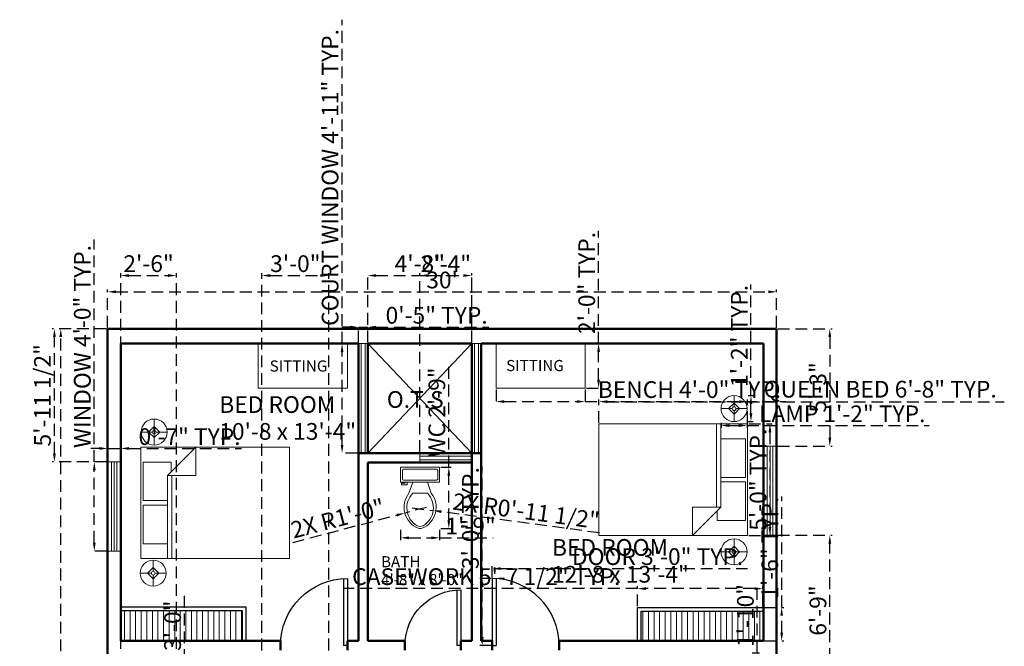
# Model space of a CAD drawing. Units: inches. Extents: x 3209 to 7144, y 1281 to 3076.
# Tile 4 of 5: x 3229 to 3758, y 1680 to 2018. Entities that reach past the tile are written whole.
import ezdxf

# ---------------------------------------------------------------- set-up
doc = ezdxf.new("R2010")
doc.units = ezdxf.units.IN
doc.linetypes.add('HIDDEN', pattern=[9.525, 6.35, -3.175])
for name, color, linetype, lineweight in [('A-ANNO-DIMS', 244, 'HIDDEN', 18), ('A-AREA-IDEN', 7, 'Continuous', 25), ('A-DOOR', 4, 'Continuous', 25), ('A-FLOR-CASE', 8, 'Continuous', 25), ('A-FLOR-CASE-PATT', 252, 'Continuous', 13), ('A-FLOR-FIXT', 9, 'Continuous', 18), ('A-FLOR-OPEN', 8, 'Continuous', 13), ('A-FURN', 8, 'Continuous', 18), ('A-GLAZ', 4, 'Continuous', 18), ('A-WALL', 7, 'Continuous', 50)]:
    doc.layers.add(name, color=color, linetype=linetype, lineweight=lineweight)
doc.styles.get("Standard").update_dxf_attribs({"font": 'arial.ttf'})
doc.dimstyles.new('ISO-25', dxfattribs={"dimtxt": 9, "dimasz": 4.5, "dimexe": 1.25, "dimexo": 0.625, "dimtad": 1, "dimdec": 0, "dimlunit": 3, "dimtxsty": 'Standard', "dimcen": 2.5, "dimadec": 0, "dimazin": 0, "dimtfac": 1, "dimtdec": 0, "dimtmove": 0, "dimatfit": 3, "dimfxl": 1, "dimarcsym": 0})

# ---------------------------------------------------------------- blocks, each defined once
blk = doc.blocks.new('Toilet - top')
for p, q in [((9.5, -6), (9.5, -2)), ((-10, -8.5), (-8, -8.5)), ((-10, -9.5), (-10, -8.5)), ((-7, -9.5), (-10, -9.5)), ((-8, -8.5), (-8, -8)), ((-7, -8), (-7, -9.5)), ((-4, -8), (-6, -14)), ((4, -8), (6, -14)), ((4, -14), (-4, -14))]:
    blk.add_line(p, q)
blk.add_lwpolyline([(10.5, -8), (10.5, 0), (-10.5, 0), (-10.5, -8)], close=True)
for points in [[(-9.5, -2), (-9.5, -6)], [(8.5, -1), (-8.5, -1)], [(-8.5, -7), (8.5, -7)]]:
    blk.add_lwpolyline(points)
for centre, radius, start, end in [((-8.62, -1.88), 0.884, 81.8699, 188.1301), ((8.62, -1.88), 0.884, 351.8699, 98.1301), ((-8.62, -6.12), 0.884, 171.8699, 278.1301), ((8.62, -6.12), 0.884, 261.8699, 8.1301), ((3.52, -21.58), 12.17, 141.4691, 247.9714), ((4.2, -21.82), 11.33, 136.3677, 238.9468), ((-3.52, -21.58), 12.17, 292.0284, 38.5307), ((-4.2, -21.82), 11.33, 301.053, 43.6321), ((0, -27.88), 4, 245.7318, 294.2682), ((0, -29), 4, 254.8605, 285.1395)]:
    blk.add_arc(centre, radius, start, end)
blk = doc.blocks.new('Bed - Queen')
for p, q in [((0, -80.00003), (0, 0)), ((0, 0), (59.99999, 0)), ((59.99999, 0), (59.99999, -80.00003)), ((7.99999, -1.2), (28.79998, -1.2)), ((7.99999, -14.4), (7.99999, -1.2)), ((28.79998, -1.2), (28.79998, -14.4)), ((31.19999, -1.2), (51.99999, -1.2)), ((31.19999, -14.4), (31.19999, -1.2)), ((51.99999, -1.2), (51.99999, -16.4)), ((0, -14.4), (44.8, -14.4)), ((59.99999, -29.6), (44.8, -14.4)), ((44.8, -14.4), (44.8, -29.6)), ((44.8, -16.8), (0, -16.8)), ((51.99999, -16.4), (46.79936, -16.4)), ((44.8, -29.6), (59.99999, -29.6)), ((59.99999, -80.00003), (0, -80.00003))]:
    blk.add_line(p, q)
blk = doc.blocks.new('Lamp - Table')
for p, q in [((0, 7), (0, 1)), ((-1, 0), (-7, 0)), ((0, 3), (-3, 0)), ((-3, 0), (0, -3)), ((3, 0), (0, 3)), ((0, -3), (3, 0)), ((1, 0), (7, 0)), ((0, -1), (0, -7))]:
    blk.add_line(p, q)
for radius in [7, 1]:
    blk.add_circle((0, 0), radius)
blk = doc.blocks.new('*D15')
at = {"layer": 'A-ANNO-DIMS', "color": 0, "lineweight": -2, "transparency": 16777216}
for p, q in [((3275.31, 1851.27), (3249.46, 1851.27)), ((3250.71, 1315.77), (3250.71, 1846.77)), ((3275.31, 1311.27), (3249.46, 1311.27))]:
    blk.add_line(p, q, dxfattribs=at)
at = {"layer": 'A-ANNO-DIMS', "color": 0, "transparency": 16777216}
for points in [[(3249.96, 1846.77), (3251.46, 1846.77), (3250.71, 1851.27)], [(3249.96, 1315.77), (3251.46, 1315.77), (3250.71, 1311.27)]]:
    blk.add_solid(points, dxfattribs=at)
at = {"layer": 'Defpoints', "color": 0, "transparency": 16777216}
for p in [(3250.71, 1851.27), (3275.94, 1851.27), (3275.94, 1311.27)]:
    blk.add_point(p, dxfattribs=at)
at = {"layer": 'A-ANNO-DIMS', "color": 0, "transparency": 16777216, "insert": (3245.51, 1581.27), "char_height": 9, "attachment_point": 5, "rotation": 90}
blk.add_mtext("45'", dxfattribs=at)
blk = doc.blocks.new('*D16')
at = {"layer": 'A-ANNO-DIMS', "color": 0, "lineweight": -2, "transparency": 16777216}
for p, q in [((3275.94, 1851.89), (3275.94, 1872.38)), ((3280.44, 1871.13), (3631.44, 1871.13)), ((3635.94, 1851.89), (3635.94, 1872.38))]:
    blk.add_line(p, q, dxfattribs=at)
at = {"layer": 'A-ANNO-DIMS', "color": 0, "transparency": 16777216}
for points in [[(3280.44, 1871.88), (3280.44, 1870.38), (3275.94, 1871.13)], [(3631.44, 1871.88), (3631.44, 1870.38), (3635.94, 1871.13)]]:
    blk.add_solid(points, dxfattribs=at)
at = {"layer": 'Defpoints', "color": 0, "transparency": 16777216}
for p in [(3635.94, 1871.13), (3275.94, 1851.27), (3635.94, 1851.27)]:
    blk.add_point(p, dxfattribs=at)
at = {"layer": 'A-ANNO-DIMS', "color": 0, "transparency": 16777216, "insert": (3455.94, 1876.35), "char_height": 9, "attachment_point": 5}
blk.add_mtext("30'", dxfattribs=at)
blk = doc.blocks.new('DOOR-SWING-36IN')
for p, q in [((0, 36), (0, 0)), ((2, 36), (2, 0)), ((0, 0), (2, 0))]:
    blk.add_line(p, q)
blk.add_arc((0, 0), 36, 0, 90)
blk = doc.blocks.new('DOOR-SWING-30IN')
for p, q in [((30, 30), (0, 30)), ((0, 30), (0, 28)), ((30, 28), (0, 28))]:
    blk.add_line(p, q)
blk.add_arc((0, 30), 30, 270, 0)
blk = doc.blocks.new('BENCH-48X24IN')
for p, q in [((0, 0), (0, 24)), ((48, 0), (48, 24)), ((0, 0), (48, 0))]:
    blk.add_line(p, q)
blk = doc.blocks.new('WINDOW-48IN-WALL7')
for p, q in [((0, 48), (7, 48)), ((2, 48), (2, 0)), ((3.5, 48), (3.5, 0)), ((5, 48), (5, 0)), ((0, 0), (7, 0))]:
    blk.add_line(p, q)
blk = doc.blocks.new('CASEWORK-BEDROOM-SURROUND')
for p, q in [((0, 67.48), (18, 67.48)), ((0, 65.48), (16, 65.48)), ((16, 65.48), (16, 0)), ((18, 67.48), (18, 0))]:
    blk.add_line(p, q)
blk = doc.blocks.new('WINDOW-LIGHTCOURT-59IN')
for p, q in [((0, 59), (5, 59)), ((1.5, 0), (1.5, 59)), ((3.5, 0), (3.5, 59))]:
    blk.add_line(p, q)
blk = doc.blocks.new('*D24')
at = {"layer": 'A-ANNO-DIMS', "color": 0, "lineweight": -2, "transparency": 16777216}
for p, q in [((3606.05, 1800.65), (3606.05, 1797.92)), ((3610.55, 1799.17), (3615.55, 1799.17)), ((3620.05, 1800.65), (3620.05, 1797.92)), ((3620.05, 1799.17), (3717.99, 1799.17))]:
    blk.add_line(p, q, dxfattribs=at)
at = {"layer": 'A-ANNO-DIMS', "color": 0, "transparency": 16777216}
for points in [[(3610.55, 1799.92), (3610.55, 1798.42), (3606.05, 1799.17)], [(3615.55, 1799.92), (3615.55, 1798.42), (3620.05, 1799.17)]]:
    blk.add_solid(points, dxfattribs=at)
at = {"layer": 'Defpoints', "color": 0, "transparency": 16777216}
for p in [(3606.05, 1801.27), (3620.05, 1801.27), (3620.05, 1799.17)]:
    blk.add_point(p, dxfattribs=at)
at = {"layer": 'A-ANNO-DIMS', "color": 0, "transparency": 16777216, "insert": (3671.27, 1804.32), "char_height": 9, "attachment_point": 5}
blk.add_mtext('LAMP 1\'-2" TYP.', dxfattribs=at)
blk = doc.blocks.new('*D25')
at = {"layer": 'A-ANNO-DIMS', "color": 0, "lineweight": -2, "transparency": 16777216}
for p, q in [((3622.15, 1815.27), (3622.15, 1875.04)), ((3620.68, 1815.27), (3623.4, 1815.27)), ((3622.15, 1805.77), (3622.15, 1810.77)), ((3620.68, 1801.27), (3623.4, 1801.27))]:
    blk.add_line(p, q, dxfattribs=at)
at = {"layer": 'A-ANNO-DIMS', "color": 0, "transparency": 16777216}
for points in [[(3621.4, 1810.77), (3622.9, 1810.77), (3622.15, 1815.27)], [(3621.4, 1805.77), (3622.9, 1805.77), (3622.15, 1801.27)]]:
    blk.add_solid(points, dxfattribs=at)
at = {"layer": 'Defpoints', "color": 0, "transparency": 16777216}
for p in [(3620.05, 1815.27), (3622.15, 1815.27), (3620.05, 1801.27)]:
    blk.add_point(p, dxfattribs=at)
at = {"layer": 'A-ANNO-DIMS', "color": 0, "transparency": 16777216, "insert": (3617.01, 1847.41), "char_height": 9, "attachment_point": 5, "rotation": 90}
blk.add_mtext('1\'-2" TYP.', dxfattribs=at)
blk = doc.blocks.new('*D27')
at = {"layer": 'A-ANNO-DIMS', "color": 0, "lineweight": -2, "transparency": 16777216}
for p, q in [((3625.56, 1676.78), (3625.56, 1712.6)), ((3622.87, 1676.78), (3626.81, 1676.78)), ((3625.56, 1659.22), (3625.56, 1672.28)), ((3622.87, 1654.72), (3626.81, 1654.72))]:
    blk.add_line(p, q, dxfattribs=at)
at = {"layer": 'A-ANNO-DIMS', "color": 0, "transparency": 16777216}
for points in [[(3624.81, 1672.28), (3626.31, 1672.28), (3625.56, 1676.78)], [(3624.81, 1659.22), (3626.31, 1659.22), (3625.56, 1654.72)]]:
    blk.add_solid(points, dxfattribs=at)
at = {"layer": 'Defpoints', "color": 0, "transparency": 16777216}
for p in [(3622.25, 1676.78), (3625.56, 1676.78), (3622.25, 1654.72)]:
    blk.add_point(p, dxfattribs=at)
at = {"layer": 'A-ANNO-DIMS', "color": 0, "transparency": 16777216, "insert": (3620.34, 1696.94), "char_height": 9, "attachment_point": 5, "rotation": 90}
blk.add_mtext('1\'-10"', dxfattribs=at)
blk = doc.blocks.new('*D30')
at = {"layer": 'A-ANNO-DIMS', "color": 0, "lineweight": -2, "transparency": 16777216}
for p, q in [((3268.74, 1779.63), (3268.74, 1899.27)), ((3275.31, 1779.63), (3267.49, 1779.63)), ((3268.74, 1736.13), (3268.74, 1775.13)), ((3275.31, 1731.63), (3267.49, 1731.63))]:
    blk.add_line(p, q, dxfattribs=at)
at = {"layer": 'A-ANNO-DIMS', "color": 0, "transparency": 16777216}
for points in [[(3267.99, 1775.13), (3269.49, 1775.13), (3268.74, 1779.63)], [(3267.99, 1736.13), (3269.49, 1736.13), (3268.74, 1731.63)]]:
    blk.add_solid(points, dxfattribs=at)
at = {"layer": 'Defpoints', "color": 0, "transparency": 16777216}
for p in [(3268.74, 1779.63), (3275.94, 1779.63), (3275.94, 1731.63)]:
    blk.add_point(p, dxfattribs=at)
at = {"layer": 'A-ANNO-DIMS', "color": 0, "transparency": 16777216, "insert": (3263.46, 1841.7), "char_height": 9, "attachment_point": 5, "rotation": 90}
blk.add_mtext('WINDOW 4\'-0" TYP.', dxfattribs=at)
blk = doc.blocks.new('*D31')
at = {"layer": 'A-ANNO-DIMS', "color": 0, "lineweight": -2, "transparency": 16777216}
for p, q in [((3271.44, 1786.83), (3266.94, 1786.83)), ((3275.94, 1780.25), (3275.94, 1788.08)), ((3275.94, 1786.83), (3282.94, 1786.83)), ((3282.94, 1780.25), (3282.94, 1788.08)), ((3287.44, 1786.83), (3348.05, 1786.83))]:
    blk.add_line(p, q, dxfattribs=at)
at = {"layer": 'A-ANNO-DIMS', "color": 0, "transparency": 16777216}
for points in [[(3271.44, 1787.58), (3271.44, 1786.08), (3275.94, 1786.83)], [(3287.44, 1787.58), (3287.44, 1786.08), (3282.94, 1786.83)]]:
    blk.add_solid(points, dxfattribs=at)
at = {"layer": 'Defpoints', "color": 0, "transparency": 16777216}
for p in [(3282.94, 1786.83), (3275.94, 1779.63), (3282.94, 1779.63)]:
    blk.add_point(p, dxfattribs=at)
at = {"layer": 'A-ANNO-DIMS', "color": 0, "transparency": 16777216, "insert": (3319.99, 1792.05), "char_height": 9, "attachment_point": 5}
blk.add_mtext('0\'-7" TYP.', dxfattribs=at)
blk = doc.blocks.new('*D32')
at = {"layer": 'A-ANNO-DIMS', "color": 0, "lineweight": -2, "transparency": 16777216}
for p, q in [((3540.36, 1800.63), (3540.36, 1813.26)), ((3620.36, 1800.63), (3620.36, 1813.26)), ((3544.86, 1812.01), (3615.86, 1812.01)), ((3620.36, 1812.01), (3758.5, 1812.01))]:
    blk.add_line(p, q, dxfattribs=at)
at = {"layer": 'A-ANNO-DIMS', "color": 0, "transparency": 16777216}
for points in [[(3544.86, 1812.76), (3544.86, 1811.26), (3540.36, 1812.01)], [(3615.86, 1812.76), (3615.86, 1811.26), (3620.36, 1812.01)]]:
    blk.add_solid(points, dxfattribs=at)
at = {"layer": 'Defpoints', "color": 0, "transparency": 16777216}
for p in [(3620.36, 1812.01), (3540.36, 1800.01), (3620.36, 1800.01)]:
    blk.add_point(p, dxfattribs=at)
at = {"layer": 'A-ANNO-DIMS', "color": 0, "transparency": 16777216, "insert": (3691.68, 1817.56), "char_height": 9, "attachment_point": 5}
blk.add_mtext('QUEEN BED 6\'-8" TYP.', dxfattribs=at)
blk = doc.blocks.new('*D33')
at = {"layer": 'A-ANNO-DIMS', "color": 0, "lineweight": -2, "transparency": 16777216}
for p, q in [((3620.98, 1800.01), (3633.61, 1800.01)), ((3632.36, 1795.51), (3632.36, 1744.51)), ((3620.98, 1740.01), (3633.61, 1740.01))]:
    blk.add_line(p, q, dxfattribs=at)
at = {"layer": 'A-ANNO-DIMS', "color": 0, "transparency": 16777216}
for points in [[(3631.61, 1795.51), (3633.11, 1795.51), (3632.36, 1800.01)], [(3631.61, 1744.51), (3633.11, 1744.51), (3632.36, 1740.01)]]:
    blk.add_solid(points, dxfattribs=at)
at = {"layer": 'Defpoints', "color": 0, "transparency": 16777216}
for p in [(3620.36, 1800.01), (3620.36, 1740.01), (3632.36, 1740.01)]:
    blk.add_point(p, dxfattribs=at)
at = {"layer": 'A-ANNO-DIMS', "color": 0, "transparency": 16777216, "insert": (3627.14, 1770.01), "char_height": 9, "attachment_point": 5, "rotation": 90}
blk.add_mtext('5\'-0" TYP.', dxfattribs=at)
blk = doc.blocks.new('*D36')
at = {"layer": 'A-ANNO-DIMS', "color": 0, "lineweight": -2, "transparency": 16777216}
for p, q in [((3482.94, 1717.39), (3482.94, 1723.42)), ((3518.94, 1717.39), (3518.94, 1723.42)), ((3487.44, 1722.17), (3514.44, 1722.17)), ((3518.94, 1722.17), (3620.31, 1722.17))]:
    blk.add_line(p, q, dxfattribs=at)
at = {"layer": 'A-ANNO-DIMS', "color": 0, "transparency": 16777216}
for points in [[(3487.44, 1722.92), (3487.44, 1721.42), (3482.94, 1722.17)], [(3514.44, 1722.92), (3514.44, 1721.42), (3518.94, 1722.17)]]:
    blk.add_solid(points, dxfattribs=at)
at = {"layer": 'Defpoints', "color": 0, "transparency": 16777216}
for p in [(3518.94, 1722.17), (3482.94, 1716.77), (3518.94, 1716.77)]:
    blk.add_point(p, dxfattribs=at)
at = {"layer": 'A-ANNO-DIMS', "color": 0, "transparency": 16777216, "insert": (3571.87, 1727.45), "char_height": 9, "attachment_point": 5}
blk.add_mtext('DOOR 3\'-0" TYP.', dxfattribs=at)
blk = doc.blocks.new('*D37')
at = {"layer": 'A-ANNO-DIMS', "color": 0, "lineweight": -2, "transparency": 16777216}
for p, q in [((3477.54, 1716.77), (3477.54, 1777.37)), ((3482.31, 1716.77), (3476.29, 1716.77)), ((3477.54, 1685.27), (3477.54, 1712.27)), ((3482.31, 1680.77), (3476.29, 1680.77))]:
    blk.add_line(p, q, dxfattribs=at)
at = {"layer": 'A-ANNO-DIMS', "color": 0, "transparency": 16777216}
for points in [[(3476.79, 1712.27), (3478.29, 1712.27), (3477.54, 1716.77)], [(3476.79, 1685.27), (3478.29, 1685.27), (3477.54, 1680.77)]]:
    blk.add_solid(points, dxfattribs=at)
at = {"layer": 'Defpoints', "color": 0, "transparency": 16777216}
for p in [(3477.54, 1716.77), (3482.94, 1716.77), (3482.94, 1680.77)]:
    blk.add_point(p, dxfattribs=at)
at = {"layer": 'A-ANNO-DIMS', "color": 0, "transparency": 16777216, "insert": (3472.32, 1749.32), "char_height": 9, "attachment_point": 5, "rotation": 90}
blk.add_mtext('3\'-0" TYP.', dxfattribs=at)
blk = doc.blocks.new('*D38')
at = {"layer": 'A-ANNO-DIMS', "color": 0, "lineweight": -2, "transparency": 16777216}
for p, q in [((3561.08, 1701.89), (3561.08, 1712.64)), ((3628.56, 1701.89), (3628.56, 1712.64)), ((3561.08, 1711.39), (3402.76, 1711.39)), ((3624.06, 1711.39), (3565.58, 1711.39))]:
    blk.add_line(p, q, dxfattribs=at)
at = {"layer": 'A-ANNO-DIMS', "color": 0, "transparency": 16777216}
for points in [[(3565.58, 1712.14), (3565.58, 1710.64), (3561.08, 1711.39)], [(3624.06, 1712.14), (3624.06, 1710.64), (3628.56, 1711.39)]]:
    blk.add_solid(points, dxfattribs=at)
at = {"layer": 'Defpoints', "color": 0, "transparency": 16777216}
for p in [(3561.08, 1711.39), (3561.08, 1701.27), (3628.56, 1701.27)]:
    blk.add_point(p, dxfattribs=at)
at = {"layer": 'A-ANNO-DIMS', "color": 0, "transparency": 16777216, "insert": (3479.67, 1716.67), "char_height": 9, "attachment_point": 5}
blk.add_mtext('CASEWORK 5\'-7 1/2" TYP.', dxfattribs=at)
blk = doc.blocks.new('*D39')
at = {"layer": 'A-ANNO-DIMS', "color": 0, "lineweight": -2, "transparency": 16777216}
for p, q in [((3638.68, 1701.27), (3638.68, 1761.03)), ((3629.19, 1701.27), (3639.93, 1701.27)), ((3638.68, 1687.77), (3638.68, 1696.77)), ((3629.19, 1683.27), (3639.93, 1683.27))]:
    blk.add_line(p, q, dxfattribs=at)
at = {"layer": 'A-ANNO-DIMS', "color": 0, "transparency": 16777216}
for points in [[(3637.93, 1696.77), (3639.43, 1696.77), (3638.68, 1701.27)], [(3637.93, 1687.77), (3639.43, 1687.77), (3638.68, 1683.27)]]:
    blk.add_solid(points, dxfattribs=at)
at = {"layer": 'Defpoints', "color": 0, "transparency": 16777216}
for p in [(3628.56, 1701.27), (3638.68, 1701.27), (3628.56, 1683.27)]:
    blk.add_point(p, dxfattribs=at)
at = {"layer": 'A-ANNO-DIMS', "color": 0, "transparency": 16777216, "insert": (3633.46, 1733.4), "char_height": 9, "attachment_point": 5, "rotation": 90}
blk.add_mtext('1\'-6" TYP.', dxfattribs=at)
blk = doc.blocks.new('*D44')
at = {"layer": 'A-ANNO-DIMS', "color": 0, "lineweight": -2, "transparency": 16777216}
for p, q in [((3484.94, 1818.64), (3484.94, 1810.82)), ((3532.94, 1818.64), (3532.94, 1810.82)), ((3489.44, 1812.07), (3528.44, 1812.07)), ((3532.94, 1812.07), (3640.66, 1812.07))]:
    blk.add_line(p, q, dxfattribs=at)
at = {"layer": 'A-ANNO-DIMS', "color": 0, "transparency": 16777216}
for points in [[(3489.44, 1812.82), (3489.44, 1811.32), (3484.94, 1812.07)], [(3528.44, 1812.82), (3528.44, 1811.32), (3532.94, 1812.07)]]:
    blk.add_solid(points, dxfattribs=at)
at = {"layer": 'Defpoints', "color": 0, "transparency": 16777216}
for p in [(3484.94, 1819.27), (3532.94, 1819.27), (3532.94, 1812.07)]:
    blk.add_point(p, dxfattribs=at)
at = {"layer": 'A-ANNO-DIMS', "color": 0, "transparency": 16777216, "insert": (3589.05, 1817.35), "char_height": 9, "attachment_point": 5}
blk.add_mtext('BENCH 4\'-0" TYP.', dxfattribs=at)
blk = doc.blocks.new('*D45')
at = {"layer": 'A-ANNO-DIMS', "color": 0, "lineweight": -2, "transparency": 16777216}
for p, q in [((3540.14, 1843.27), (3540.14, 1904.03)), ((3533.57, 1843.27), (3541.39, 1843.27)), ((3540.14, 1823.77), (3540.14, 1838.77)), ((3533.57, 1819.27), (3541.39, 1819.27))]:
    blk.add_line(p, q, dxfattribs=at)
at = {"layer": 'A-ANNO-DIMS', "color": 0, "transparency": 16777216}
for points in [[(3539.39, 1838.77), (3540.89, 1838.77), (3540.14, 1843.27)], [(3539.39, 1823.77), (3540.89, 1823.77), (3540.14, 1819.27)]]:
    blk.add_solid(points, dxfattribs=at)
at = {"layer": 'Defpoints', "color": 0, "transparency": 16777216}
for p in [(3532.94, 1843.27), (3540.14, 1843.27), (3532.94, 1819.27)]:
    blk.add_point(p, dxfattribs=at)
at = {"layer": 'A-ANNO-DIMS', "color": 0, "transparency": 16777216, "insert": (3534.92, 1875.9), "char_height": 9, "attachment_point": 5, "rotation": 90}
blk.add_mtext('2\'-0" TYP.', dxfattribs=at)
blk = doc.blocks.new('*D48')
at = {"layer": 'A-ANNO-DIMS', "color": 0, "lineweight": -2, "transparency": 16777216}
for p, q in [((3402.09, 1843.27), (3402.09, 2017.62)), ((3410.31, 1843.27), (3400.84, 1843.27)), ((3402.09, 1788.77), (3402.09, 1838.77)), ((3410.31, 1784.27), (3400.84, 1784.27))]:
    blk.add_line(p, q, dxfattribs=at)
at = {"layer": 'A-ANNO-DIMS', "color": 0, "transparency": 16777216}
for points in [[(3401.34, 1838.77), (3402.84, 1838.77), (3402.09, 1843.27)], [(3401.34, 1788.77), (3402.84, 1788.77), (3402.09, 1784.27)]]:
    blk.add_solid(points, dxfattribs=at)
at = {"layer": 'Defpoints', "color": 0, "transparency": 16777216}
for p in [(3402.09, 1843.27), (3410.94, 1843.27), (3410.94, 1784.27)]:
    blk.add_point(p, dxfattribs=at)
at = {"layer": 'A-ANNO-DIMS', "color": 0, "transparency": 16777216, "insert": (3396.81, 1932.69), "char_height": 9, "attachment_point": 5, "rotation": 90}
blk.add_mtext('COURT WINDOW 4\'-11" TYP.', dxfattribs=at)
blk = doc.blocks.new('*D49')
at = {"layer": 'A-ANNO-DIMS', "color": 0, "lineweight": -2, "transparency": 16777216}
for p, q in [((3406.44, 1852.12), (3401.94, 1852.12)), ((3410.94, 1843.89), (3410.94, 1853.37)), ((3410.94, 1852.12), (3415.94, 1852.12)), ((3415.94, 1843.89), (3415.94, 1853.37)), ((3420.44, 1852.12), (3481.05, 1852.12))]:
    blk.add_line(p, q, dxfattribs=at)
at = {"layer": 'A-ANNO-DIMS', "color": 0, "transparency": 16777216}
for points in [[(3406.44, 1852.87), (3406.44, 1851.37), (3410.94, 1852.12)], [(3420.44, 1852.87), (3420.44, 1851.37), (3415.94, 1852.12)]]:
    blk.add_solid(points, dxfattribs=at)
at = {"layer": 'Defpoints', "color": 0, "transparency": 16777216}
for p in [(3415.94, 1852.12), (3410.94, 1843.27), (3415.94, 1843.27)]:
    blk.add_point(p, dxfattribs=at)
at = {"layer": 'A-ANNO-DIMS', "color": 0, "transparency": 16777216, "insert": (3452.99, 1857.34), "char_height": 9, "attachment_point": 5}
blk.add_mtext('0\'-5" TYP.', dxfattribs=at)
blk = doc.blocks.new('*D50')
at = {"layer": 'A-ANNO-DIMS', "color": 0, "lineweight": -2, "transparency": 16777216}
for p, q in [((3459.55, 1776.72), (3459.55, 1831.21)), ((3455.22, 1776.72), (3460.8, 1776.72)), ((3459.55, 1748.18), (3459.55, 1772.22)), ((3455.22, 1743.68), (3460.8, 1743.68))]:
    blk.add_line(p, q, dxfattribs=at)
at = {"layer": 'A-ANNO-DIMS', "color": 0, "transparency": 16777216}
for points in [[(3458.8, 1772.22), (3460.3, 1772.22), (3459.55, 1776.72)], [(3458.8, 1748.18), (3460.3, 1748.18), (3459.55, 1743.68)]]:
    blk.add_solid(points, dxfattribs=at)
at = {"layer": 'Defpoints', "color": 0, "transparency": 16777216}
for p in [(3454.59, 1776.72), (3459.55, 1776.72), (3454.59, 1743.68)]:
    blk.add_point(p, dxfattribs=at)
at = {"layer": 'A-ANNO-DIMS', "color": 0, "transparency": 16777216, "insert": (3454.27, 1806.21), "char_height": 9, "attachment_point": 5, "rotation": 90}
blk.add_mtext('WC 2\'-9"', dxfattribs=at)
blk = doc.blocks.new('*D51')
at = {"layer": 'A-ANNO-DIMS', "color": 0, "lineweight": -2, "transparency": 16777216}
for p, q in [((3433.59, 1743.05), (3433.59, 1737.47)), ((3438.09, 1738.72), (3450.09, 1738.72)), ((3454.59, 1743.05), (3454.59, 1737.47)), ((3454.59, 1738.72), (3483.42, 1738.72))]:
    blk.add_line(p, q, dxfattribs=at)
at = {"layer": 'A-ANNO-DIMS', "color": 0, "transparency": 16777216}
for points in [[(3438.09, 1739.47), (3438.09, 1737.97), (3433.59, 1738.72)], [(3450.09, 1739.47), (3450.09, 1737.97), (3454.59, 1738.72)]]:
    blk.add_solid(points, dxfattribs=at)
at = {"layer": 'Defpoints', "color": 0, "transparency": 16777216}
for p in [(3433.59, 1743.68), (3454.59, 1743.68), (3454.59, 1738.72)]:
    blk.add_point(p, dxfattribs=at)
at = {"layer": 'A-ANNO-DIMS', "color": 0, "transparency": 16777216, "insert": (3471.26, 1743.94), "char_height": 9, "attachment_point": 5}
blk.add_mtext('1\'-9"', dxfattribs=at)
blk = doc.blocks.new('*D60')
at = {"layer": 'A-ANNO-DIMS', "color": 0, "lineweight": -2, "transparency": 16777216}
for p, q in [((3317.34, 1577.27), (3317.34, 1709.86)), ((3312.56, 1577.27), (3318.59, 1577.27)), ((3317.34, 1545.77), (3317.34, 1572.77)), ((3312.56, 1541.27), (3318.59, 1541.27))]:
    blk.add_line(p, q, dxfattribs=at)
at = {"layer": 'A-ANNO-DIMS', "color": 0, "transparency": 16777216}
for points in [[(3316.59, 1572.77), (3318.09, 1572.77), (3317.34, 1577.27)], [(3316.59, 1545.77), (3318.09, 1545.77), (3317.34, 1541.27)]]:
    blk.add_solid(points, dxfattribs=at)
at = {"layer": 'Defpoints', "color": 0, "transparency": 16777216}
for p in [(3311.94, 1577.27), (3317.34, 1577.27), (3311.94, 1541.27)]:
    blk.add_point(p, dxfattribs=at)
at = {"layer": 'A-ANNO-DIMS', "color": 0, "transparency": 16777216, "insert": (3312.05, 1645.82), "char_height": 9, "attachment_point": 5, "rotation": 90}
blk.add_mtext('REFRIGERATOR 3\'-0"', dxfattribs=at)
blk = doc.blocks.new('*D74')
at = {"layer": 'A-ANNO-DIMS', "color": 0, "lineweight": -2, "transparency": 16777216}
for p, q in [((3282.94, 1678.89), (3282.94, 1881.16)), ((3312.94, 1678.89), (3312.94, 1881.16)), ((3287.44, 1879.91), (3308.44, 1879.91))]:
    blk.add_line(p, q, dxfattribs=at)
at = {"layer": 'A-ANNO-DIMS', "color": 0, "transparency": 16777216}
for points in [[(3287.44, 1880.66), (3287.44, 1879.16), (3282.94, 1879.91)], [(3308.44, 1880.66), (3308.44, 1879.16), (3312.94, 1879.91)]]:
    blk.add_solid(points, dxfattribs=at)
at = {"layer": 'Defpoints', "color": 0, "transparency": 16777216}
for p in [(3312.94, 1879.91), (3282.94, 1678.27), (3312.94, 1678.27)]:
    blk.add_point(p, dxfattribs=at)
at = {"layer": 'A-ANNO-DIMS', "color": 0, "transparency": 16777216, "insert": (3297.94, 1885.14), "char_height": 9, "attachment_point": 5}
blk.add_mtext('2\'-6"', dxfattribs=at)
blk = doc.blocks.new('*D75')
at = {"layer": 'A-ANNO-DIMS', "color": 0, "lineweight": -2, "transparency": 16777216}
for p, q in [((3358.94, 1582.89), (3358.94, 1881.16)), ((3394.94, 1582.89), (3394.94, 1881.16)), ((3363.44, 1879.91), (3390.44, 1879.91))]:
    blk.add_line(p, q, dxfattribs=at)
at = {"layer": 'A-ANNO-DIMS', "color": 0, "transparency": 16777216}
for points in [[(3363.44, 1880.66), (3363.44, 1879.16), (3358.94, 1879.91)], [(3390.44, 1880.66), (3390.44, 1879.16), (3394.94, 1879.91)]]:
    blk.add_solid(points, dxfattribs=at)
at = {"layer": 'Defpoints', "color": 0, "transparency": 16777216}
for p in [(3394.94, 1879.91), (3358.94, 1582.27), (3394.94, 1582.27)]:
    blk.add_point(p, dxfattribs=at)
at = {"layer": 'A-ANNO-DIMS', "color": 0, "transparency": 16777216, "insert": (3376.94, 1885.14), "char_height": 9, "attachment_point": 5}
blk.add_mtext('3\'-0"', dxfattribs=at)
blk = doc.blocks.new('*D76')
at = {"layer": 'A-ANNO-DIMS', "color": 0, "lineweight": -2, "transparency": 16777216}
for p, q in [((3415.94, 1843.89), (3415.94, 1881.16)), ((3471.94, 1843.89), (3471.94, 1881.16)), ((3420.44, 1879.91), (3467.44, 1879.91))]:
    blk.add_line(p, q, dxfattribs=at)
at = {"layer": 'A-ANNO-DIMS', "color": 0, "transparency": 16777216}
for points in [[(3420.44, 1880.66), (3420.44, 1879.16), (3415.94, 1879.91)], [(3467.44, 1880.66), (3467.44, 1879.16), (3471.94, 1879.91)]]:
    blk.add_solid(points, dxfattribs=at)
at = {"layer": 'Defpoints', "color": 0, "transparency": 16777216}
for p in [(3471.94, 1879.91), (3415.94, 1843.27), (3471.94, 1843.27)]:
    blk.add_point(p, dxfattribs=at)
at = {"layer": 'A-ANNO-DIMS', "color": 0, "transparency": 16777216, "insert": (3443.94, 1885.14), "char_height": 9, "attachment_point": 5}
blk.add_mtext('4\'-8"', dxfattribs=at)
blk = doc.blocks.new('*D77')
at = {"layer": 'A-ANNO-DIMS', "color": 0, "lineweight": -2, "transparency": 16777216}
for p, q in [((3443.94, 1784.89), (3443.94, 1881.16)), ((3471.94, 1784.89), (3471.94, 1881.16)), ((3448.44, 1879.91), (3467.44, 1879.91))]:
    blk.add_line(p, q, dxfattribs=at)
at = {"layer": 'A-ANNO-DIMS', "color": 0, "transparency": 16777216}
for points in [[(3448.44, 1880.66), (3448.44, 1879.16), (3443.94, 1879.91)], [(3467.44, 1880.66), (3467.44, 1879.16), (3471.94, 1879.91)]]:
    blk.add_solid(points, dxfattribs=at)
at = {"layer": 'Defpoints', "color": 0, "transparency": 16777216}
for p in [(3471.94, 1879.91), (3443.94, 1784.27), (3471.94, 1784.27)]:
    blk.add_point(p, dxfattribs=at)
at = {"layer": 'A-ANNO-DIMS', "color": 0, "transparency": 16777216, "insert": (3457.94, 1885.06), "char_height": 9, "attachment_point": 5}
blk.add_mtext('2\'-4"', dxfattribs=at)
blk = doc.blocks.new('*D78')
at = {"layer": 'A-ANNO-DIMS', "color": 0, "lineweight": -2, "transparency": 16777216}
for p, q in [((3636.56, 1851.27), (3665.83, 1851.27)), ((3664.58, 1846.77), (3664.58, 1792.63)), ((3636.56, 1788.13), (3665.83, 1788.13))]:
    blk.add_line(p, q, dxfattribs=at)
at = {"layer": 'A-ANNO-DIMS', "color": 0, "transparency": 16777216}
for points in [[(3663.83, 1846.77), (3665.33, 1846.77), (3664.58, 1851.27)], [(3663.83, 1792.63), (3665.33, 1792.63), (3664.58, 1788.13)]]:
    blk.add_solid(points, dxfattribs=at)
at = {"layer": 'Defpoints', "color": 0, "transparency": 16777216}
for p in [(3635.94, 1851.27), (3635.94, 1788.13), (3664.58, 1788.13)]:
    blk.add_point(p, dxfattribs=at)
at = {"layer": 'A-ANNO-DIMS', "color": 0, "transparency": 16777216, "insert": (3659.36, 1819.7), "char_height": 9, "attachment_point": 5, "rotation": 90}
blk.add_mtext('5\'-3"', dxfattribs=at)
blk = doc.blocks.new('*D79')
at = {"layer": 'A-ANNO-DIMS', "color": 0, "lineweight": -2, "transparency": 16777216}
for p, q in [((3636.56, 1740.13), (3665.83, 1740.13)), ((3664.58, 1663.54), (3664.58, 1735.63)), ((3636.56, 1659.04), (3665.83, 1659.04))]:
    blk.add_line(p, q, dxfattribs=at)
at = {"layer": 'A-ANNO-DIMS', "color": 0, "transparency": 16777216}
for points in [[(3663.83, 1735.63), (3665.33, 1735.63), (3664.58, 1740.13)], [(3663.83, 1663.54), (3665.33, 1663.54), (3664.58, 1659.04)]]:
    blk.add_solid(points, dxfattribs=at)
at = {"layer": 'Defpoints', "color": 0, "transparency": 16777216}
for p in [(3635.94, 1740.13), (3664.58, 1740.13), (3635.94, 1659.04)]:
    blk.add_point(p, dxfattribs=at)
at = {"layer": 'A-ANNO-DIMS', "color": 0, "transparency": 16777216, "insert": (3659.36, 1699.59), "char_height": 9, "attachment_point": 5, "rotation": 90}
blk.add_mtext('6\'-9"', dxfattribs=at)
blk = doc.blocks.new('*D81')
at = {"layer": 'A-ANNO-DIMS', "color": 0, "lineweight": -2, "transparency": 16777216}
for p, q in [((3275.31, 1851.27), (3246.04, 1851.27)), ((3247.29, 1784.13), (3247.29, 1846.77)), ((3275.31, 1779.63), (3246.04, 1779.63))]:
    blk.add_line(p, q, dxfattribs=at)
at = {"layer": 'A-ANNO-DIMS', "color": 0, "transparency": 16777216}
for points in [[(3246.54, 1846.77), (3248.04, 1846.77), (3247.29, 1851.27)], [(3246.54, 1784.13), (3248.04, 1784.13), (3247.29, 1779.63)]]:
    blk.add_solid(points, dxfattribs=at)
at = {"layer": 'Defpoints', "color": 0, "transparency": 16777216}
for p in [(3247.29, 1851.27), (3275.94, 1851.27), (3275.94, 1779.63)]:
    blk.add_point(p, dxfattribs=at)
at = {"layer": 'A-ANNO-DIMS', "color": 0, "transparency": 16777216, "insert": (3242.01, 1815.45), "char_height": 9, "attachment_point": 5, "rotation": 90}
blk.add_mtext('5\'-11 1/2"', dxfattribs=at)
blk = doc.blocks.new('*D86')
at = {"layer": 'A-ANNO-DIMS', "color": 0, "lineweight": -2, "transparency": 16777216}
for p, q in [((3447.61, 1755.14), (3435.84, 1752.05)), ((3375.61, 1736.22), (3431.49, 1750.91))]:
    blk.add_line(p, q, dxfattribs=at)
at = {"layer": 'A-ANNO-DIMS', "color": 0, "transparency": 16777216}
blk.add_solid([(3431.3, 1751.63), (3431.68, 1750.18), (3435.84, 1752.05)], dxfattribs=at)
at = {"layer": 'Defpoints', "color": 0, "transparency": 16777216}
for p in [(3447.61, 1755.14), (3435.84, 1752.05)]:
    blk.add_point(p, dxfattribs=at)
at = {"layer": 'A-ANNO-DIMS', "color": 0, "transparency": 16777216, "insert": (3400.05, 1748.04), "char_height": 9, "attachment_point": 5, "rotation": 14.7213}
blk.add_mtext('2X R1\'-0"', dxfattribs=at)
blk = doc.blocks.new('*D87')
at = {"layer": 'A-ANNO-DIMS', "color": 0, "lineweight": -2, "transparency": 16777216}
for p, q in [((3439.89, 1754.91), (3451.12, 1753.4)), ((3540.56, 1741.37), (3455.58, 1752.8))]:
    blk.add_line(p, q, dxfattribs=at)
at = {"layer": 'A-ANNO-DIMS', "color": 0, "transparency": 16777216}
blk.add_solid([(3455.68, 1753.54), (3455.48, 1752.05), (3451.12, 1753.4)], dxfattribs=at)
at = {"layer": 'Defpoints', "color": 0, "transparency": 16777216}
for p in [(3439.89, 1754.91), (3451.12, 1753.4)]:
    blk.add_point(p, dxfattribs=at)
at = {"layer": 'A-ANNO-DIMS', "color": 0, "transparency": 16777216, "insert": (3501, 1752.02), "char_height": 9, "attachment_point": 5, "rotation": 352.3429}
blk.add_mtext('2X R0\'-11 1/2"', dxfattribs=at)

msp = doc.modelspace()

# ---------------------------------------------------------------- hatches: boundary and pattern name
at = {"layer": 'A-FLOR-CASE-PATT'}
h = msp.add_hatch(dxfattribs=at)
h.set_pattern_fill('ANSI31', color=256, scale=0.944882, angle=45, style=0)
h.paths.add_polyline_path([(3282.42, 1683.42), (3348.42, 1683.42), (3348.42, 1699.42), (3282.42, 1699.42)])
h = msp.add_hatch(dxfattribs=at)
h.set_pattern_fill('ANSI31', color=256, scale=0.944882, angle=45, style=0)
h.paths.add_polyline_path([(3563.08, 1683.27), (3628.56, 1683.27), (3628.56, 1699.27), (3563.08, 1699.27)])

# ---------------------------------------------------------------- linework, layer by layer
at = {"layer": 'A-FLOR-OPEN'}
for p, q in [((3415.94, 1843.27), (3471.94, 1784.27)), ((3415.94, 1784.27), (3471.94, 1843.27))]:
    msp.add_line(p, q, dxfattribs=at)
at = {"layer": 'A-GLAZ'}
for p, q in [((3443.94, 1784.27), (3443.94, 1779.27)), ((3443.94, 1782.77), (3471.94, 1782.77)), ((3443.94, 1780.77), (3471.94, 1780.77))]:
    msp.add_line(p, q, dxfattribs=at)
at = {"layer": 'A-WALL'}
for p, q in [((3275.94, 1851.27), (3635.94, 1851.27)), ((3275.94, 1311.27), (3275.94, 1851.27)), ((3635.94, 1851.27), (3635.94, 1311.27)), ((3282.94, 1843.27), (3410.94, 1843.27)), ((3282.94, 1683.27), (3282.94, 1843.27)), ((3410.94, 1683.27), (3410.94, 1843.27)), ((3415.94, 1784.27), (3415.94, 1843.27)), ((3415.94, 1843.27), (3471.94, 1843.27)), ((3471.94, 1843.27), (3471.94, 1779.27)), ((3476.94, 1843.27), (3476.94, 1683.27)), ((3476.94, 1843.27), (3628.94, 1843.27)), ((3628.94, 1843.27), (3628.94, 1683.27)), ((3410.94, 1784.27), (3476.94, 1784.27)), ((3415.94, 1683.27), (3415.94, 1779.27)), ((3415.94, 1779.27), (3471.94, 1779.27)), ((3471.94, 1779.27), (3471.94, 1683.27)), ((3282.94, 1683.27), (3368.94, 1683.27)), ((3368.94, 1678.27), (3368.94, 1683.27)), ((3404.94, 1683.27), (3410.94, 1683.27)), ((3404.94, 1678.27), (3404.94, 1683.27)), ((3415.94, 1683.27), (3435.94, 1683.27)), ((3435.94, 1683.27), (3435.94, 1678.27)), ((3465.94, 1683.27), (3465.94, 1678.27)), ((3465.94, 1683.27), (3471.94, 1683.27)), ((3476.94, 1683.27), (3482.94, 1683.27)), ((3482.94, 1683.27), (3482.94, 1678.27)), ((3518.94, 1683.27), (3518.94, 1678.27)), ((3518.94, 1683.27), (3628.94, 1683.27))]:
    msp.add_line(p, q, dxfattribs=at)

# ---------------------------------------------------------------- block references
at = {"layer": 'A-DOOR', "extrusion": (0, 0, -1), "zscale": -1}
msp.add_blockref('DOOR-SWING-36IN', (-3404.94, 1680.77), dxfattribs=at)
at = {"layer": 'A-DOOR'}
msp.add_blockref('DOOR-SWING-36IN', (3482.94, 1680.77), dxfattribs=at)
at = {"layer": 'A-DOOR', "extrusion": (0, 0, -1), "zscale": -1, "rotation": 90.0000000000039}
msp.add_blockref('DOOR-SWING-30IN', (-3435.94, 1680.77), dxfattribs=at)
at = {"layer": 'A-FLOR-CASE', "extrusion": (0, 0, -1), "zscale": -1, "rotation": 90.00000000000026}
msp.add_blockref('CASEWORK-BEDROOM-SURROUND', (-3282.94, 1683.42), dxfattribs=at)
at = {"layer": 'A-FLOR-CASE', "rotation": 90.00000000000055}
msp.add_blockref('CASEWORK-BEDROOM-SURROUND', (3628.56, 1683.27), dxfattribs=at)
at = {"layer": 'A-FLOR-FIXT'}
msp.add_blockref('Toilet - top', (3444.09, 1776.72), dxfattribs=at)
at = {"layer": 'A-FURN'}
for name, p in [('BENCH-48X24IN', (3356.94, 1819.27)), ('BENCH-48X24IN', (3484.94, 1819.27)), ('Lamp - Table', (3613.05, 1808.27)), ('Lamp - Table', (3300.97, 1795.66)), ('Lamp - Table', (3613.05, 1731.19)), ('Lamp - Table', (3300.45, 1719.7))]:
    msp.add_blockref(name, p, dxfattribs=at)
for p, rotation in [((3620.36, 1800.01), 270), ((3293.76, 1727.54), 90)]:
    msp.add_blockref('Bed - Queen', p, dxfattribs=dict(at, rotation=rotation))
at = {"layer": 'A-GLAZ'}
for name, p in [('WINDOW-LIGHTCOURT-59IN', (3410.94, 1784.27)), ('WINDOW-LIGHTCOURT-59IN', (3471.94, 1784.27)), ('WINDOW-48IN-WALL7', (3628.94, 1740.13)), ('WINDOW-48IN-WALL7', (3275.94, 1731.63))]:
    msp.add_blockref(name, p, dxfattribs=at)

# ---------------------------------------------------------------- texts
at = {"layer": 'A-AREA-IDEN'}
for s, height, p in [('SITTING ', 6, (3363.12, 1828.21)), ('SITTING ', 6, (3490.4, 1828.46)), ('O.T.S', 9, (3426.17, 1808.7)), ('BED ROOM ', 9, (3336, 1805.97)), ('10\'-8 x 13\'-4"', 9, (3336, 1791.51)), ('BED ROOM ', 9, (3515.07, 1729.07)), ('BATH', 6, (3423.05, 1722.87)), ('12\'-8 x 13\'-4"', 9, (3515.07, 1714.61)), ('4\'-8" x 8\'-0"', 6, (3423.05, 1713.24))]:
    msp.add_text(s, height=height, dxfattribs=at).set_placement(p)

# ---------------------------------------------------------------- dimensions: what is measured, and where the dimension line sits
at = {"layer": 'A-ANNO-DIMS'}
for base, p1, p2, angle, text, picture, middle in [((3402.09, 1843.27), (3410.94, 1784.27), (3410.94, 1843.27), 90, 'COURT WINDOW <> TYP.', '*D48', (3396.81, 1932.69)), ((3540.14, 1843.27), (3532.94, 1819.27), (3532.94, 1843.27), 90, '<> TYP.', '*D45', (3534.92, 1875.9)), ((3268.74, 1779.63), (3275.94, 1731.63), (3275.94, 1779.63), 90, 'WINDOW <> TYP.', '*D30', (3263.46, 1841.7)), ((3622.15, 1815.27), (3620.05, 1801.27), (3620.05, 1815.27), 90, '<> TYP.', '*D25', (3617.01, 1847.41)), ((3459.55, 1776.72), (3454.59, 1743.68), (3454.59, 1776.72), 90, 'WC <>', '*D50', (3454.27, 1806.21)), ((3632.36, 1740.01), (3620.36, 1800.01), (3620.36, 1740.01), 270, '<> TYP.', '*D33', (3627.14, 1770.01)), ((3477.54, 1716.77), (3482.94, 1680.77), (3482.94, 1716.77), 90, '<> TYP.', '*D37', (3472.32, 1749.32)), ((3638.68, 1701.27), (3628.56, 1683.27), (3628.56, 1701.27), 90, '<> TYP.', '*D39', (3633.46, 1733.4)), ((3561.08, 1711.39), (3628.56, 1701.27), (3561.08, 1701.27), 180, 'CASEWORK <> TYP.', '*D38', (3479.67, 1716.67)), ((3317.34, 1577.27), (3311.94, 1541.27), (3311.94, 1577.27), 90, 'REFRIGERATOR <>', '*D60', (3312.05, 1645.82))]:
    dim = msp.add_linear_dim(base=base, p1=p1, p2=p2, angle=angle, text=text, dimstyle='ISO-25', override={"dimdec": 1, "dimlfac": 1, "dimrnd": 0, "dimzin": 1, "dimdsep": 46, "dimlunit": 4, "dimfrac": 2}, dxfattribs=at)
    dim.commit()
    dim.dimension.update_dxf_attribs({"geometry": picture, "text_midpoint": middle})
for base, p1, p2, override, picture, middle in [((3312.94, 1879.91), (3282.94, 1678.27), (3312.94, 1678.27), {"dimdec": 1, "dimlfac": 1, "dimrnd": 0, "dimzin": 1, "dimdsep": 46, "dimlunit": 4, "dimfrac": 2}, '*D74', (3297.94, 1885.14)), ((3394.94, 1879.91), (3358.94, 1582.27), (3394.94, 1582.27), {"dimdec": 1, "dimlfac": 1, "dimrnd": 0, "dimzin": 1, "dimdsep": 46, "dimlunit": 4, "dimfrac": 2}, '*D75', (3376.94, 1885.14)), ((3471.94, 1879.91), (3415.94, 1843.27), (3471.94, 1843.27), {"dimdec": 1, "dimlfac": 1, "dimrnd": 0, "dimzin": 1, "dimdsep": 46, "dimlunit": 4, "dimfrac": 2}, '*D76', (3443.94, 1885.14)), ((3471.94, 1879.91), (3443.94, 1784.27), (3471.94, 1784.27), {"dimdec": 1, "dimlfac": 1, "dimrnd": 0, "dimzin": 1, "dimdsep": 46, "dimlunit": 4, "dimfrac": 2}, '*D77', (3457.94, 1885.06)), ((3635.94, 1871.13), (3275.94, 1851.27), (3635.94, 1851.27), {"dimclrd": 0, "dimclre": 0, "dimclrt": 0}, '*D16', (3455.94, 1876.35)), ((3454.59, 1738.72), (3433.59, 1743.68), (3454.59, 1743.68), {"dimdec": 1, "dimlfac": 1, "dimrnd": 0, "dimzin": 1, "dimdsep": 46, "dimlunit": 4, "dimfrac": 2}, '*D51', (3471.26, 1743.94))]:
    dim = msp.add_linear_dim(base=base, p1=p1, p2=p2, dimstyle='ISO-25', override=override, dxfattribs=at)
    dim.commit()
    dim.dimension.update_dxf_attribs({"geometry": picture, "text_midpoint": middle})
for base, p1, p2, text, picture, middle in [((3415.94, 1852.12), (3410.94, 1843.27), (3415.94, 1843.27), '<> TYP.', '*D49', (3452.99, 1857.34)), ((3620.36, 1812.01), (3540.36, 1800.01), (3620.36, 1800.01), 'QUEEN BED <> TYP.', '*D32', (3691.68, 1817.56)), ((3532.94, 1812.07), (3484.94, 1819.27), (3532.94, 1819.27), 'BENCH <> TYP.', '*D44', (3589.05, 1817.35)), ((3620.05, 1799.17), (3606.05, 1801.27), (3620.05, 1801.27), 'LAMP <> TYP.', '*D24', (3671.27, 1804.32)), ((3282.94, 1786.83), (3275.94, 1779.63), (3282.94, 1779.63), '<> TYP.', '*D31', (3319.99, 1792.05)), ((3518.94, 1722.17), (3482.94, 1716.77), (3518.94, 1716.77), 'DOOR <> TYP.', '*D36', (3571.87, 1727.45))]:
    dim = msp.add_linear_dim(base=base, p1=p1, p2=p2, text=text, dimstyle='ISO-25', override={"dimdec": 1, "dimlfac": 1, "dimrnd": 0, "dimzin": 1, "dimdsep": 46, "dimlunit": 4, "dimfrac": 2}, dxfattribs=at)
    dim.commit()
    dim.dimension.update_dxf_attribs({"geometry": picture, "text_midpoint": middle})
for base, p1, p2, override, picture, middle in [((3247.29, 1851.27), (3275.94, 1779.63), (3275.94, 1851.27), {"dimdec": 1, "dimlfac": 1, "dimrnd": 0, "dimzin": 1, "dimdsep": 46, "dimlunit": 4, "dimfrac": 2}, '*D81', (3242.01, 1815.45)), ((3250.71, 1851.27), (3275.94, 1311.27), (3275.94, 1851.27), {"dimclrd": 0, "dimclre": 0, "dimclrt": 0}, '*D15', (3245.51, 1581.27)), ((3664.58, 1788.13), (3635.94, 1851.27), (3635.94, 1788.13), {"dimdec": 1, "dimlfac": 1, "dimrnd": 0, "dimzin": 1, "dimdsep": 46, "dimlunit": 4, "dimfrac": 2}, '*D78', (3659.36, 1819.7)), ((3664.58, 1740.13), (3635.94, 1659.04), (3635.94, 1740.13), {"dimdec": 1, "dimlfac": 1, "dimrnd": 0, "dimzin": 1, "dimdsep": 46, "dimlunit": 4, "dimfrac": 2}, '*D79', (3659.36, 1699.59)), ((3625.56, 1676.78), (3622.25, 1654.72), (3622.25, 1676.78), {"dimdec": 1, "dimlfac": 1, "dimrnd": 0, "dimzin": 1, "dimdsep": 46, "dimlunit": 4, "dimfrac": 2}, '*D27', (3620.34, 1696.94))]:
    dim = msp.add_linear_dim(base=base, p1=p1, p2=p2, angle=90, dimstyle='ISO-25', override=override, dxfattribs=at)
    dim.commit()
    dim.dimension.update_dxf_attribs({"geometry": picture, "text_midpoint": middle})
for center, mpoint, picture, middle in [((3439.89, 1754.91), (3451.12, 1753.4), '*D87', (3501, 1752.02)), ((3447.61, 1755.14), (3435.84, 1752.05), '*D86', (3400.05, 1748.04))]:
    dim = msp.add_radius_dim(center=center, mpoint=mpoint, text='2X <>', dimstyle='ISO-25', override={"dimdec": 1, "dimlfac": 1, "dimrnd": 0, "dimzin": 1, "dimdsep": 46, "dimlunit": 4, "dimfrac": 2}, dxfattribs=at)
    dim.commit()
    dim.dimension.update_dxf_attribs({"geometry": picture, "text_midpoint": middle})

doc.saveas('drawing.dxf')
